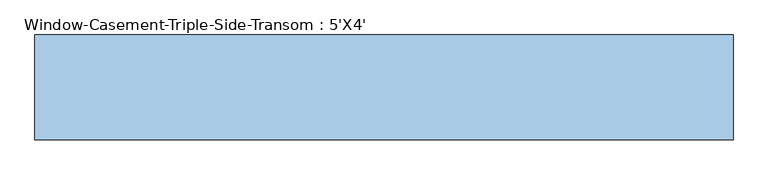
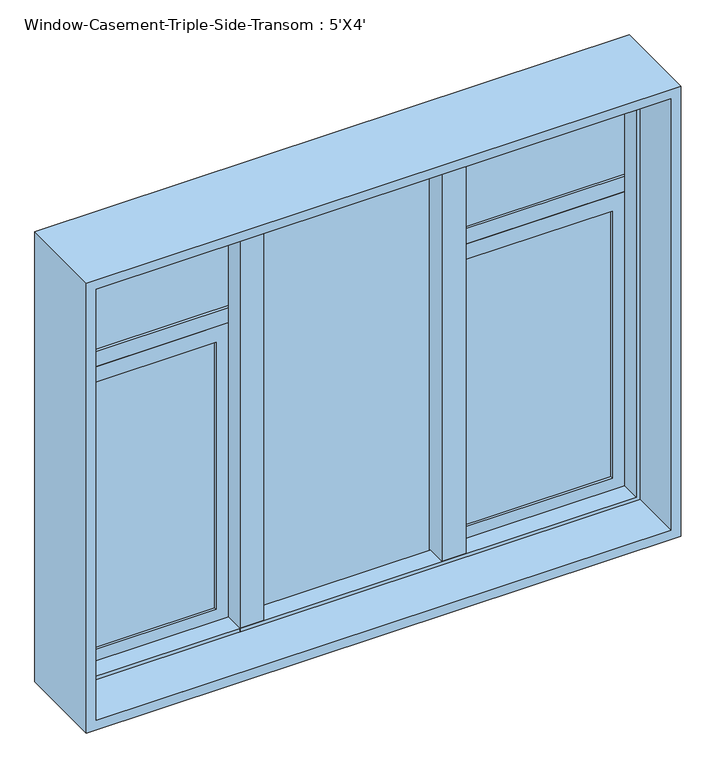
"""IFC4 building model written with IfcOpenShell, lengths in millimetres: window geometry, Window-Casement-Triple-Side-Transom : 5'X4'."""

from ifc_helpers import new_model, si_unit, frame, origin, place, context, project, spatial, polyline, outline, extrude, faceted_brep, source, transform, mapped, element, save


def window_casement_triple_side_transom_5_x4_f59ddf0b(model_context):
    return source(origin(), model_context, "Body", "SolidModel", [
        faceted_brep([(-736.6, 73.025, 2108.2), (-736.6, 114.3, 2108.2), (736.6, 114.3, 2108.2), (736.6, 73.025, 2108.2), (-726.4796875, 22.225, 2098.0796875), (-726.4796875, 73.025, 2098.0796875), (726.4796875, 73.025, 2098.0796875), (726.4796875, 22.225, 2098.0796875), (-736.6, -114.3, 2108.2), (-736.6, 22.225, 2108.2), (736.6, 22.225, 2108.2), (736.6, -114.3, 2108.2), (-762.0, 114.3, 2133.6), (-762.0, -114.3, 2133.6), (762.0, -114.3, 2133.6), (762.0, 114.3, 2133.6), (736.6, 114.3, 939.8), (736.6, 73.025, 939.8), (726.4796875, 73.025, 949.9203125), (726.4796875, 22.225, 949.9203125), (736.6, 22.225, 939.8), (736.6, -114.3, 939.8), (762.0, -114.3, 914.4), (762.0, 114.3, 914.4), (-736.6, 114.3, 939.8), (-736.6, 73.025, 939.8), (-726.4796875, 73.025, 949.9203125), (-726.4796875, 22.225, 949.9203125), (-736.6, 22.225, 939.8), (-736.6, -114.3, 939.8), (-762.0, -114.3, 914.4), (-762.0, 114.3, 914.4)], [[[0, 1, 2, 3]], [[4, 5, 6, 7]], [[8, 9, 10, 11]], [[12, 13, 14, 15]], [[3, 2, 16, 17]], [[7, 6, 18, 19]], [[11, 10, 20, 21]], [[15, 14, 22, 23]], [[17, 16, 24, 25]], [[19, 18, 26, 27]], [[21, 20, 28, 29]], [[23, 22, 30, 31]], [[25, 24, 1, 0]], [[3, 17, 25, 0], [5, 26, 18, 6]], [[27, 26, 5, 4]], [[9, 28, 20, 10], [7, 19, 27, 4]], [[29, 28, 9, 8]], [[13, 30, 22, 14], [11, 21, 29, 8]], [[31, 30, 13, 12]], [[15, 23, 31, 12], [1, 24, 16, 2]]]),
        extrude(outline(polyline([(-228.6, 111.125), (-228.6, 22.225), (-289.5203125, 22.225), (-289.5203125, 73.025), (-279.4, 73.025), (-279.4, 111.125), (-228.6, 111.125)])), frame((0.0, 0.0, 939.8), z_axis=(0.0, 0.0, 1.0), x_axis=(1.0, 0.0, 0.0)), (0.0, 0.0, 1.0), 1168.4),
        extrude(outline(polyline([(279.4, 111.125), (279.4, 73.025), (289.5203125, 73.025), (289.5203125, 22.225), (228.6, 22.225), (228.6, 111.125), (279.4, 111.125)])), frame((0.0, 0.0, 939.8), z_axis=(0.0, 0.0, 1.0), x_axis=(1.0, 0.0, 0.0)), (0.0, 0.0, 1.0), 1168.4),
        extrude(outline(polyline([(1746.9048438, 279.4), (939.8, 279.4), (939.8, 736.6), (1746.9048438, 736.6), (1746.9048438, 279.4)]), holes=[polyline([(1705.0345313, 694.7296875), (981.6703125, 694.7296875), (981.6703125, 321.2703125), (1705.0345313, 321.2703125), (1705.0345313, 694.7296875)])]), frame((0.0, 73.025, 0.0), z_axis=(0.0, 1.0, 0.0), x_axis=(0.0, 0.0, 1.0)), (0.0, 0.0, 1.0), 31.75),
        extrude(outline(polyline([(1746.9048438, -736.6), (939.8, -736.6), (939.8, -279.4), (1746.9048438, -279.4), (1746.9048438, -736.6)]), holes=[polyline([(1705.0345313, -321.2703125), (981.6703125, -321.2703125), (981.6703125, -694.7296875), (1705.0345313, -694.7296875), (1705.0345313, -321.2703125)])]), frame((0.0, 73.025, 0.0), z_axis=(0.0, 1.0, 0.0), x_axis=(0.0, 0.0, 1.0)), (0.0, 0.0, 1.0), 31.75),
        extrude(outline(polyline([(-321.2703125, 98.425), (-321.2703125, 92.075), (-694.7296875, 92.075), (-694.7296875, 98.425), (-321.2703125, 98.425)])), frame((0.0, 0.0, 981.6703125), z_axis=(0.0, 0.0, 1.0), x_axis=(1.0, 0.0, 0.0)), (0.0, 0.0, 1.0), 723.3642188),
        extrude(outline(polyline([(-321.2703125, 85.725), (-321.2703125, 79.375), (-694.7296875, 79.375), (-694.7296875, 85.725), (-321.2703125, 85.725)])), frame((0.0, 0.0, 981.6703125), z_axis=(0.0, 0.0, 1.0), x_axis=(1.0, 0.0, 0.0)), (0.0, 0.0, 1.0), 723.3642188),
        extrude(outline(polyline([(694.7296875, 98.425), (694.7296875, 92.075), (321.2703125, 92.075), (321.2703125, 98.425), (694.7296875, 98.425)])), frame((0.0, 0.0, 981.6703125), z_axis=(0.0, 0.0, 1.0), x_axis=(1.0, 0.0, 0.0)), (0.0, 0.0, 1.0), 723.3642188),
        extrude(outline(polyline([(694.7296875, 85.725), (694.7296875, 79.375), (321.2703125, 79.375), (321.2703125, 85.725), (694.7296875, 85.725)])), frame((0.0, 0.0, 981.6703125), z_axis=(0.0, 0.0, 1.0), x_axis=(1.0, 0.0, 0.0)), (0.0, 0.0, 1.0), 723.3642188),
        extrude(outline(polyline([(736.6, 104.775), (736.6, 73.025), (279.4, 73.025), (279.4, 104.775), (736.6, 104.775)])), frame((0.0, 0.0, 1746.9048438), z_axis=(0.0, 0.0, 1.0), x_axis=(1.0, 0.0, 0.0)), (0.0, 0.0, 1.0), 41.8703125),
        extrude(outline(polyline([(228.6, 98.425), (228.6, 92.075), (-228.6, 92.075), (-228.6, 98.425), (228.6, 98.425)])), frame((0.0, 0.0, 939.8), z_axis=(0.0, 0.0, 1.0), x_axis=(1.0, 0.0, 0.0)), (0.0, 0.0, 1.0), 1168.4),
        extrude(outline(polyline([(228.6, 85.725), (228.6, 79.375), (-228.6, 79.375), (-228.6, 85.725), (228.6, 85.725)])), frame((0.0, 0.0, 939.8), z_axis=(0.0, 0.0, 1.0), x_axis=(1.0, 0.0, 0.0)), (0.0, 0.0, 1.0), 1168.4),
        extrude(outline(polyline([(-279.4, 104.775), (-279.4, 73.025), (-736.6, 73.025), (-736.6, 104.775), (-279.4, 104.775)])), frame((0.0, 0.0, 1746.9048438), z_axis=(0.0, 0.0, 1.0), x_axis=(1.0, 0.0, 0.0)), (0.0, 0.0, 1.0), 41.8703125),
        extrude(outline(polyline([(-279.4, 98.425), (-279.4, 92.075), (-736.6, 92.075), (-736.6, 98.425), (-279.4, 98.425)])), frame((0.0, 0.0, 1788.7751562), z_axis=(0.0, 0.0, 1.0), x_axis=(1.0, 0.0, 0.0)), (0.0, 0.0, 1.0), 319.4248438),
        extrude(outline(polyline([(-279.4, 85.725), (-279.4, 79.375), (-736.6, 79.375), (-736.6, 85.725), (-279.4, 85.725)])), frame((0.0, 0.0, 1788.7751562), z_axis=(0.0, 0.0, 1.0), x_axis=(1.0, 0.0, 0.0)), (0.0, 0.0, 1.0), 319.4248438),
        extrude(outline(polyline([(736.6, 98.425), (736.6, 92.075), (279.4, 92.075), (279.4, 98.425), (736.6, 98.425)])), frame((0.0, 0.0, 1788.7751562), z_axis=(0.0, 0.0, 1.0), x_axis=(1.0, 0.0, 0.0)), (0.0, 0.0, 1.0), 319.4248438),
        extrude(outline(polyline([(736.6, 85.725), (736.6, 79.375), (279.4, 79.375), (279.4, 85.725), (736.6, 85.725)])), frame((0.0, 0.0, 1788.7751562), z_axis=(0.0, 0.0, 1.0), x_axis=(1.0, 0.0, 0.0)), (0.0, 0.0, 1.0), 319.4248438),
    ])


if __name__ == "__main__":
    model = new_model("IFC4")
    model_context = context("Model", 3, world=origin())
    ifc_project = project(units=[si_unit("LENGTHUNIT", "METRE", prefix="MILLI")], contexts=[model_context])
    site = spatial("IfcSite", under=ifc_project)
    building = spatial("IfcBuilding", under=site)
    placement = place(None, origin())
    window_casement_triple_side_transom_5_x4_shape = window_casement_triple_side_transom_5_x4_f59ddf0b(model_context)
    element("IfcWindow", 1, ObjectType="Window-Casement-Triple-Side-Transom : 5'X4'", at=placement, inside=building, context=model_context, shape_type="MappedRepresentation", body=[
        mapped(window_casement_triple_side_transom_5_x4_shape, transform((0.0, 0.0, 0.0), x_axis=(1.0, 0.0, 0.0), y_axis=(0.0, 1.0, 0.0), z_axis=(0.0, 0.0, 1.0))),
    ])
    save(model, "model.ifc")

# Revit data of these elements
# Type "Window-Casement-Triple-Side-Transom : 5'X4'"
#   Type Mark = "24"
#   Fire Rating = "0.5h"
#   Assembly Code = "B2020100"
#   Analytic Construction = "Double glazing - domestic"
#   Window Width = 1' - 8"
#   Window Inset [instance default] = 0' - 0 5/8"
#   Wall Thickness [instance default] = 0' - 6"
#   Visual Light Transmittance = 0.81
#   Transom Height Ratio = 0.3
#   Thermal Resistance (R) = 1.8146 (h·ft²·°F)/BTU
#   Solar Heat Gain Coefficient = 0.76
#   Rough Width = 5' - 0 1/2"
#   Rough Height = 4' - 0 1/2"
#   Open Window Height = 2' - 9.6"
#   Heat Transfer Coefficient (U) = 0.5511 BTU/(h·ft²·°F)
#   Height = 4' - 0"
#   Transom Height = 1' - 2.4"
#   Frame Gap 3 [instance default] = 0' - 1 83/128"
#   Frame Gap 2 [instance default] = 0' - 0 5/8"
#   Frame Gap 1 = 0' - 1 51/128"
#   Default Sill Height = 3' - 0"
#   Width = 5' - 0"
#   Frame Material = Metal - Aluminum
#   Glass Panel Material = Glass
#   Wall Closure = (empty or 0)
# Element 1 (IfcWindow, "Window-Casement-Triple-Side-Transom : 5'X4'")
#   Wall Thickness = 0' - 9"
#   Materials on its faces: "Metal - Aluminum", "Glass"
# Materials
#   "Metal - Aluminum": class "Metal", colour RGB 247 247 247, transparency 0
#   "Glass": class "Glass", colour RGB 0 128 192, transparency 0.75, Description = "Soda Lime Glass", Cost = 0
